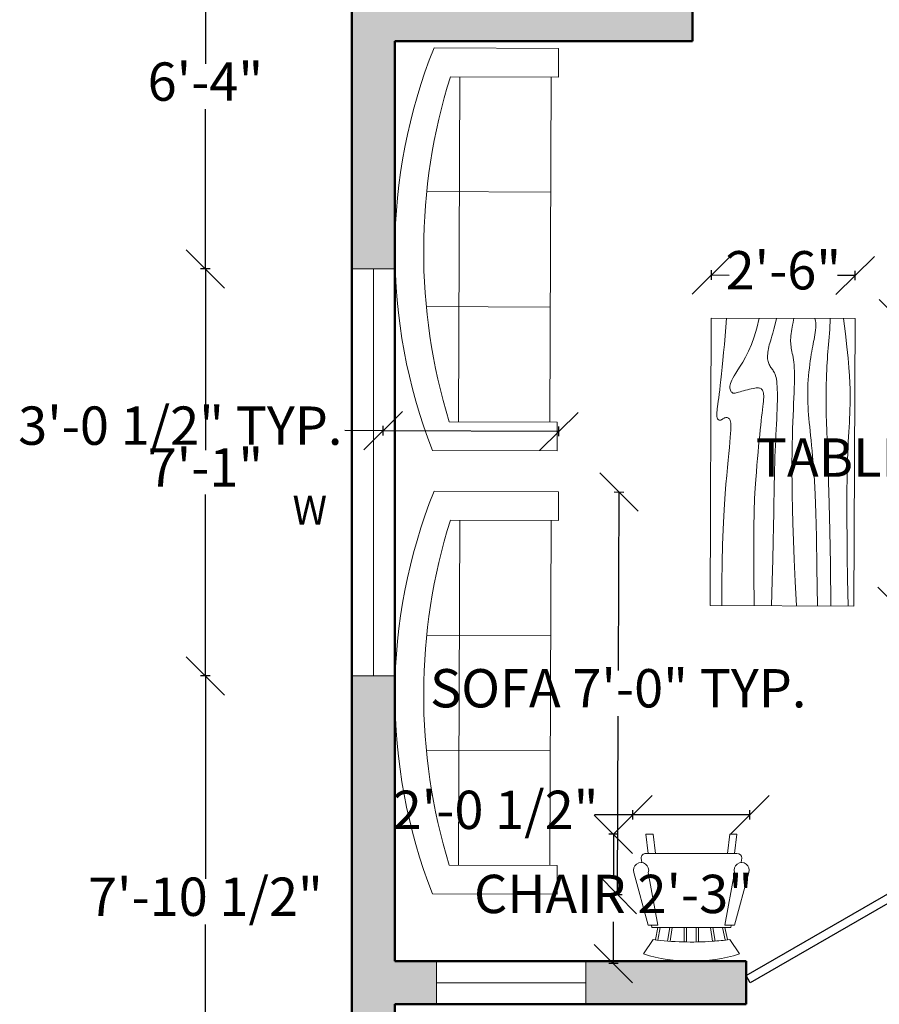
# Model space of a CAD drawing. Units: inches. Extents: x 3121 to 3511, y 1323 to 1998.
# Tile 7 of 10: x 3121 to 3300, y 1539 to 1744. Entities that reach past the tile are written whole.
import ezdxf

# ---------------------------------------------------------------- set-up
doc = ezdxf.new("R2010")
doc.units = ezdxf.units.IN
for name, color, linetype, lineweight in [('A-ANNO-DIMS', 2, 'Continuous', 18), ('A-ANNO-TEXT', 7, 'Continuous', 18), ('A-DOOR', 3, 'Continuous', 25), ('A-FURN', 8, 'Continuous', 18), ('A-GLAZ', 4, 'Continuous', 18), ('A-WALL', 7, 'Continuous', 50), ('A-WALL-PATT', 3, 'Continuous', 13)]:
    doc.layers.add(name, color=color, linetype=linetype, lineweight=lineweight)
doc.styles.get("Standard").update_dxf_attribs({"font": 'arial.ttf'})
doc.dimstyles.new('ISO-25', dxfattribs={"dimtxt": 8, "dimasz": 8, "dimexe": 1, "dimexo": 1, "dimtad": 0, "dimtih": 1, "dimtoh": 1, "dimlunit": 3, "dimtxsty": 'Standard', "dimblk": 'OBLIQUE', "dimcen": 2.5, "dimclrt": 1, "dimadec": 0, "dimazin": 0, "dimtfac": 1, "dimtmove": 0, "dimatfit": 3, "dimfxl": 1, "dimfxlon": 1, "dimarcsym": 0})

# ---------------------------------------------------------------- blocks, each defined once
blk = doc.blocks.new('Chair - Rocking')
for p, q in [((-8, -4.5), (-10, -1.5)), ((8, -4.5), (10, -1.5)), ((-1.5, -4.05012), (-1.5, -7)), ((-1, -7), (-1, -4.05012)), ((1, -7), (1, -4.04655)), ((1.5, -4.05012), (1.5, -7)), ((-7.5, -4.5), (-7, -7)), ((-6.5, -7), (-7.02225, -4.43)), ((-4.5, -7), (-4.96674, -4.19951)), ((-4, -7), (-4.40532, -4.16272)), ((4, -7), (4.40187, -4.18694)), ((4.5, -7), (4.96761, -4.19437)), ((6.5, -7), (7, -4.4057)), ((7.5, -4.5), (7, -7)), ((-9, -7.5), (-12, -18.49999)), ((-7, -7.5), (-9, -7.5)), ((-9, -18.49999), (-7, -7.5)), ((-8.23428, -6.99939), (-8.3093, -7.47958)), ((-8.23041, -7), (8.23915, -7)), ((7, -7.5), (9, -7.5)), ((9, -18.49999), (7, -7.5)), ((8.31071, -7.48854), (8.23449, -7.00073)), ((9, -7.5), (12, -18.49999)), ((-10.36644, -20.64523), (-10.5, -21.49999)), ((-9, -22.49999), (-9.5, -26.49999)), ((0, -22.49999), (-9.5, -22.49999)), ((-8, -26.49999), (-7.5, -22.49999)), ((0, -22.49999), (9.5, -22.49999)), ((8, -26.49999), (7.5, -22.49999)), ((9, -22.49999), (9.5, -26.49999)), ((10.5, -21.49999), (10.3575, -20.58798)), ((-9.5, -26.49999), (-8, -26.49999)), ((9.5, -26.49999), (8, -26.49999))]:
    blk.add_line(p, q)
for centre, radius, start, end in [((0, -34.08333), 34.08333, 72.93847, 107.0615), ((0, -68.25004), 64.25, 82.84733, 93.92211), ((0, -68.25004), 64.25, 93.92211, 97.15267), ((-10.5, -18.99999), 1.58114, 161.5651, 18.43495), ((10.5, -18.99999), 1.58114, 161.5651, 18.43495), ((-9.5, -21.49999), 1, 180, 270), ((9.5, -21.49999), 1, 270, 0)]:
    blk.add_arc(centre, radius, start, end)
blk = doc.blocks.new('Sofa - Roundback 7 ft.')
for p, q in [((-12.00002, -32.4421), (-12.00003, -6.5971)), ((11.99997, -32.4421), (11.99998, -6.5971)), ((-36.000027, -34), (-36.000027, -11.4696)), ((35.99998, -34), (35.99998, -11.4696)), ((-35.999844, -13.3819), (35.9998, -13.3819)), ((-36.000027, -32.4421), (35.99998, -32.4421))]:
    blk.add_line(p, q)
for points in [[(-36.000027, -34), (-42.000027, -34), (-42.000027, -8)], [(41.99998, -8), (41.99998, -34), (35.99998, -34)]]:
    blk.add_lwpolyline(points)
for centre, radius, start, end in [((0, -114.25), 114.25, 68.43141, 111.5686), ((-0.00001, -127.1968), 121.1968, 72.72033, 107.2797)]:
    blk.add_arc(centre, radius, start, end)
blk = doc.blocks.new('Table - Rectangular Woodgrain 60 x 30 in.')
for p, q in [((0, 0), (0, -30)), ((60, 0), (0, 0)), ((60, -30), (60, 0)), ((0, -30), (60, -30))]:
    blk.add_line(p, q)
for points in [[(0, -2.4), (4.8155, -2.418), (9.0302, -2.4688), (12.709, -2.5477), (15.9167, -2.65), (18.7181, -2.7711), (21.1781, -2.9063), (23.3616, -3.0508), (25.3333, -3.2), (27.1477, -3.3495), (28.8172, -3.4958), (30.3437, -3.636), (31.7291, -3.7667), (32.9756, -3.8849), (34.0849, -3.9875), (35.059, -4.0714), (35.9, -4.1334), (36.6114, -4.1711), (37.2041, -4.1854), (37.6906, -4.1779), (38.0833, -4.15), (38.3948, -4.1034), (38.6375, -4.0396), (38.8239, -3.9602), (38.9666, -3.8667), (39.0764, -3.7608), (39.1573, -3.6448), (39.2116, -3.521), (39.2416, -3.3917), (39.2498, -3.2593), (39.2385, -3.1261), (39.21, -2.9944), (39.1666, -2.8667), (39.111, -2.7447), (39.0468, -2.6281), (38.978, -2.5163), (38.9083, -2.4083), (38.8418, -2.3035), (38.7823, -2.201), (38.7337, -2.1001), (38.7, -2), (38.6844, -1.9003), (38.6875, -1.8021), (38.7094, -1.707), (38.75, -1.6167), (38.8094, -1.5326), (38.8875, -1.4563), (38.9844, -1.3893), (39.1, -1.3333), (39.2351, -1.2896), (39.3937, -1.2583), (39.5804, -1.2396), (39.8, -1.2333), (40.057, -1.2396), (40.3562, -1.2583), (40.7023, -1.2896), (41.1, -1.3333), (41.5547, -1.3895), (42.0755, -1.4573), (42.6721, -1.5361), (43.3542, -1.625), (44.1316, -1.7233), (45.014, -1.8302), (46.0114, -1.9449), (47.1333, -2.0667), (48.3862, -2.1947), (49.7625, -2.3281), (51.2513, -2.4663), (52.8416, -2.6083), (54.5226, -2.7535), (56.2833, -2.9011), (58.1127, -3.0501), (60, -3.2)], [(0, -9.2), (6.5759, -9.0858), (11.9385, -9.0365), (16.2527, -9.0418), (19.6833, -9.0917), (22.3952, -9.1759), (24.5531, -9.2844), (26.322, -9.4069), (27.8666, -9.5333), (29.3241, -9.6553), (30.7203, -9.7719), (32.0532, -9.8837), (33.3208, -9.9917), (34.5213, -10.0965), (35.6526, -10.199), (36.7128, -10.2999), (37.7, -10.4), (38.6129, -10.4996), (39.4531, -10.5969), (40.223, -10.6895), (40.925, -10.775), (41.5613, -10.8512), (42.1344, -10.9156), (42.6465, -10.966), (43.1, -11), (43.4976, -11.0158), (43.8437, -11.0136), (44.143, -10.9942), (44.4, -10.9583), (44.6195, -10.9069), (44.8062, -10.8406), (44.9648, -10.7603), (45.1, -10.6667), (45.2155, -10.5598), (45.3114, -10.4365), (45.3871, -10.2929), (45.4416, -10.125), (45.4743, -9.929), (45.4844, -9.7011), (45.4709, -9.4371), (45.4333, -9.1333), (45.3716, -8.7883), (45.2896, -8.4104), (45.1919, -8.0107), (45.0833, -7.6), (44.9685, -7.1893), (44.8521, -6.7896), (44.7388, -6.4117), (44.6333, -6.0667), (44.54, -5.7628), (44.4614, -5.4979), (44.4001, -5.2675), (44.3583, -5.0667), (44.3384, -4.8909), (44.3427, -4.7354), (44.3736, -4.5956), (44.4333, -4.4667), (44.5236, -4.3453), (44.6427, -4.2333), (44.7884, -4.1339), (44.9583, -4.05), (45.1501, -3.9849), (45.3614, -3.9417), (45.59, -3.9234), (45.8333, -3.9333), (46.0915, -3.9749), (46.3734, -4.0531), (46.6906, -4.1736), (47.0542, -4.3417), (47.4756, -4.5629), (47.9661, -4.8427), (48.5372, -5.1866), (49.2, -5.6), (49.9676, -6.0844), (50.8594, -6.625), (51.8965, -7.2031), (53.1, -7.8), (54.491, -8.3969), (56.0906, -8.975), (57.9199, -9.5156), (60, -10)], [(0, -12.8), (5.1847, -12.9322), (9.6213, -13.0323), (13.3963, -13.1059), (16.5958, -13.1583), (19.3063, -13.1952), (21.614, -13.2219), (23.6054, -13.2439), (25.3666, -13.2667), (26.9728, -13.2947), (28.4531, -13.3281), (29.8256, -13.3663), (31.1083, -13.4083), (32.3191, -13.4535), (33.476, -13.501), (34.597, -13.5501), (35.7, -13.6), (36.7984, -13.6497), (37.8875, -13.6979), (38.9578, -13.743), (40, -13.7833), (41.0047, -13.8174), (41.9625, -13.8438), (42.864, -13.8607), (43.7, -13.8667), (44.4631, -13.8604), (45.1552, -13.8417), (45.7801, -13.8104), (46.3416, -13.7667), (46.8439, -13.7104), (47.2906, -13.6417), (47.6858, -13.5604), (48.0333, -13.4667), (48.3375, -13.3608), (48.6042, -13.2448), (48.8396, -13.121), (49.05, -12.9917), (49.2417, -12.8593), (49.4208, -12.7261), (49.5937, -12.5944), (49.7667, -12.4667), (49.9452, -12.3451), (50.1323, -12.2313), (50.3303, -12.1268), (50.5416, -12.0333), (50.7686, -11.9524), (51.0135, -11.8854), (51.2788, -11.8341), (51.5666, -11.8), (51.8785, -11.7843), (52.2116, -11.7865), (52.562, -11.8059), (52.926, -11.8417), (53.2998, -11.8931), (53.6795, -11.9594), (54.0614, -12.0397), (54.4416, -12.1333), (54.8223, -12.2401), (55.2293, -12.3625), (55.6942, -12.5037), (56.2489, -12.6667), (56.9251, -12.8547), (57.7545, -13.0708), (58.7689, -13.3182), (60, -13.6)], [(0, -18), (5.124, -17.7273), (9.6609, -17.5057), (13.6705, -17.3303), (17.2125, -17.1958), (20.3467, -17.0973), (23.1328, -17.0297), (25.6307, -16.9878), (27.9, -16.9667), (29.9928, -16.9617), (31.9302, -16.9703), (33.7254, -16.9907), (35.3917, -17.0208), (36.9423, -17.0588), (38.3906, -17.1026), (39.7499, -17.1503), (41.0333, -17.2), (42.2519, -17.2496), (43.4073, -17.2969), (44.4986, -17.3395), (45.525, -17.375), (46.4858, -17.4012), (47.3802, -17.4156), (48.2074, -17.416), (48.9667, -17.4), (49.6583, -17.3662), (50.2872, -17.3167), (50.8595, -17.2547), (51.3812, -17.1833), (51.8584, -17.1057), (52.2971, -17.025), (52.7034, -16.9443), (53.0833, -16.8667), (53.443, -16.7951), (53.789, -16.7313), (54.128, -16.6768), (54.4666, -16.6334), (54.8115, -16.6024), (55.1693, -16.5854), (55.5465, -16.5841), (55.95, -16.6), (56.3828, -16.6337), (56.8346, -16.6823), (57.2915, -16.7418), (57.7396, -16.8084), (58.165, -16.878), (58.5539, -16.9469), (58.8924, -17.0111), (59.1666, -17.0667), (59.3679, -17.1107), (59.5078, -17.1438), (59.6032, -17.1675), (59.6708, -17.1833), (59.7275, -17.193), (59.7901, -17.1979), (59.8753, -17.1998), (60, -17.2)], [(0, -22.4), (8.0098, -22.2501), (14.4094, -22.1011), (19.4168, -21.9535), (23.25, -21.8083), (26.1269, -21.6663), (28.2656, -21.5281), (29.884, -21.3947), (31.2, -21.2667), (32.3967, -21.1448), (33.5172, -21.0292), (34.5697, -20.9198), (35.5625, -20.8167), (36.5037, -20.7198), (37.4015, -20.6292), (38.2642, -20.5448), (39.1, -20.4667), (39.9164, -20.3951), (40.7187, -20.3313), (41.5117, -20.2768), (42.3, -20.2333), (43.0883, -20.2024), (43.8812, -20.1854), (44.6836, -20.1841), (45.5, -20.2), (46.3328, -20.234), (47.1747, -20.2844), (48.0163, -20.3488), (48.8479, -20.425), (49.66, -20.5106), (50.4429, -20.6031), (51.1872, -20.7004), (51.8833, -20.8), (52.5246, -20.8999), (53.1166, -20.9995), (53.6681, -21.0983), (54.1875, -21.1958), (54.6834, -21.2919), (55.1646, -21.3859), (55.6394, -21.4777), (56.1167, -21.5667), (56.6028, -21.6515), (57.0961, -21.7266), (57.5929, -21.7852), (58.0896, -21.8208), (58.5823, -21.8268), (59.0674, -21.7964), (59.5412, -21.723), (60, -21.6)], [(0, -25.2), (8.6355, -25.0504), (15.7026, -24.9031), (21.4049, -24.7606), (25.9458, -24.625), (29.529, -24.4988), (32.3578, -24.3844), (34.6359, -24.284), (36.5667, -24.2), (38.3213, -24.1341), (39.9417, -24.0854), (41.437, -24.0523), (42.8167, -24.0333), (44.0901, -24.0268), (45.2667, -24.0313), (46.3557, -24.0451), (47.3667, -24.0667), (48.309, -24.0947), (49.1928, -24.1287), (50.0284, -24.168), (50.826, -24.2125), (51.5959, -24.2617), (52.3483, -24.3151), (53.0935, -24.3725), (53.8417, -24.4334), (54.6009, -24.497), (55.3699, -24.561), (56.1454, -24.6226), (56.9239, -24.6792), (57.7021, -24.7279), (58.4764, -24.7662), (59.2435, -24.7911), (60, -24.8)], [(0, -28.8), (5.6867, -28.6681), (10.45, -28.5698), (14.407, -28.5012), (17.675, -28.4584), (20.3711, -28.4374), (22.6125, -28.4344), (24.5164, -28.4455), (26.2, -28.4667), (27.762, -28.4947), (29.2276, -28.5281), (30.6033, -28.5663), (31.8958, -28.6084), (33.1118, -28.6535), (34.2578, -28.7011), (35.3405, -28.7501), (36.3666, -28.8), (37.3443, -28.8497), (38.288, -28.8974), (39.2137, -28.9412), (40.1375, -28.9792), (41.0753, -29.0093), (42.0432, -29.0297), (43.0572, -29.0384), (44.1333, -29.0333), (45.2936, -29.0114), (46.5843, -28.9641), (48.0579, -28.8816), (49.7666, -28.7542), (51.7629, -28.5721), (54.0989, -28.3255), (56.8272, -28.0048), (60, -27.6)]]:
    blk.add_lwpolyline(points)
blk = doc.blocks.new('*U11')
for p, q in [((0, 0), (0, -6)), ((40, 0), (40, -6))]:
    blk.add_line(p, q)
blk.add_lwpolyline([(0, 0), (34.64, 20), (35.52, 18.48), (0.87, -1.52)], close=True)
blk.add_arc((0, 0), 40, 0, 30)
blk = doc.blocks.new('_Oblique')
at = {"color": 0, "linetype": 'ByBlock', "lineweight": -2}
blk.add_line((-0.5, -0.5), (0.5, 0.5), dxfattribs=at)
blk = doc.blocks.new('*D21')
at = {"layer": 'A-ANNO-DIMS', "color": 0, "lineweight": -2, "transparency": 16777216}
for p, q in [((3244.67, 1645.71), (3246.67, 1645.7)), ((3245.67, 1645.71), (3245.54, 1608.47)), ((3245.36, 1561.71), (3245.5, 1598.94)), ((3244.36, 1561.71), (3246.36, 1561.7))]:
    blk.add_line(p, q, dxfattribs=at)
at = {"layer": 'Defpoints', "color": 0, "transparency": 16777216}
for p in [(3233.07, 1645.75), (3245.67, 1645.71), (3232.76, 1561.76)]:
    blk.add_point(p, dxfattribs=at)
at = {"layer": 'A-ANNO-DIMS', "color": 0, "lineweight": -2, "transparency": 16777216, "xscale": 8, "yscale": 8, "zscale": 8}
for p, rotation in [((3245.67, 1645.71), 89.78583340711933), ((3245.36, 1561.71), 269.7858334071193)]:
    blk.add_blockref('_Oblique', p, dxfattribs=dict(at, rotation=rotation))
at = {"layer": 'A-ANNO-DIMS', "color": 1, "transparency": 16777216, "insert": (3245.52, 1603.71), "char_height": 8, "attachment_point": 5}
blk.add_mtext('SOFA 7\'-0" TYP.', dxfattribs=at)
blk = doc.blocks.new('*D22')
at = {"layer": 'A-ANNO-DIMS', "color": 0, "lineweight": -2, "transparency": 16777216}
for p, q in [((3196.46, 1658.49), (3188.46, 1658.52)), ((3196.45, 1657.49), (3196.46, 1659.49)), ((3233.12, 1658.35), (3196.46, 1658.49)), ((3233.12, 1657.35), (3233.13, 1659.35))]:
    blk.add_line(p, q, dxfattribs=at)
at = {"layer": 'Defpoints', "color": 0, "transparency": 16777216}
for p in [(3196.46, 1658.49), (3196.41, 1645.89), (3233.07, 1645.75)]:
    blk.add_point(p, dxfattribs=at)
at = {"layer": 'A-ANNO-DIMS', "color": 0, "lineweight": -2, "transparency": 16777216, "xscale": 8, "yscale": 8, "zscale": 8}
for p, rotation in [((3196.46, 1658.49), 179.7858334071193), ((3233.12, 1658.35), 359.7858334071194)]:
    blk.add_blockref('_Oblique', p, dxfattribs=dict(at, rotation=rotation))
at = {"layer": 'A-ANNO-DIMS', "color": 1, "transparency": 16777216, "insert": (3154.13, 1658.52), "char_height": 8, "attachment_point": 5}
blk.add_mtext('3\'-0 1/2" TYP.', dxfattribs=at)
blk = doc.blocks.new('*D25')
at = {"layer": 'A-ANNO-DIMS', "color": 0, "lineweight": -2, "transparency": 16777216}
for p, q in [((3245.53, 1574.28), (3243.53, 1574.28)), ((3244.53, 1574.28), (3244.53, 1565.55)), ((3244.53, 1547.28), (3244.53, 1556.02)), ((3245.53, 1547.28), (3243.53, 1547.28))]:
    blk.add_line(p, q, dxfattribs=at)
at = {"layer": 'Defpoints', "color": 0, "transparency": 16777216}
for p in [(3248.58, 1574.28), (3244.53, 1547.28), (3248.58, 1547.28)]:
    blk.add_point(p, dxfattribs=at)
at = {"layer": 'A-ANNO-DIMS', "color": 0, "lineweight": -2, "transparency": 16777216, "xscale": 8, "yscale": 8, "zscale": 8}
for p, rotation in [((3244.53, 1574.28), 90), ((3244.53, 1547.28), 270)]:
    blk.add_blockref('_Oblique', p, dxfattribs=dict(at, rotation=rotation))
at = {"layer": 'A-ANNO-DIMS', "color": 1, "transparency": 16777216, "insert": (3244.53, 1560.78), "char_height": 8, "attachment_point": 5}
blk.add_mtext('CHAIR 2\'-3"', dxfattribs=at)
blk = doc.blocks.new('*D26')
at = {"layer": 'A-ANNO-DIMS', "color": 0, "lineweight": -2, "transparency": 16777216}
for p, q in [((3248.58, 1578.33), (3240.58, 1578.33)), ((3248.58, 1577.33), (3248.58, 1579.33)), ((3273.01, 1578.33), (3248.58, 1578.33)), ((3273.01, 1577.33), (3273.01, 1579.33))]:
    blk.add_line(p, q, dxfattribs=at)
at = {"layer": 'Defpoints', "color": 0, "transparency": 16777216}
for p in [(3248.58, 1578.33), (3248.58, 1574.28), (3273.01, 1574.28)]:
    blk.add_point(p, dxfattribs=at)
at = {"layer": 'A-ANNO-DIMS', "color": 0, "lineweight": -2, "transparency": 16777216, "xscale": 8, "yscale": 8, "zscale": 8, "rotation": 180}
blk.add_blockref('_Oblique', (3248.58, 1578.33), dxfattribs=at)
at = {"layer": 'A-ANNO-DIMS', "color": 0, "lineweight": -2, "transparency": 16777216, "xscale": 8, "yscale": 8, "zscale": 8}
blk.add_blockref('_Oblique', (3273.01, 1578.33), dxfattribs=at)
at = {"layer": 'A-ANNO-DIMS', "color": 1, "transparency": 16777216, "insert": (3219.93, 1578.33), "char_height": 8, "attachment_point": 5}
blk.add_mtext('2\'-0 1/2"', dxfattribs=at)
blk = doc.blocks.new('*D29')
at = {"layer": 'A-ANNO-DIMS', "color": 0, "lineweight": -2, "transparency": 16777216}
for p, q in [((3302.93, 1681.86), (3304.93, 1681.86)), ((3303.93, 1681.86), (3303.84, 1656.57)), ((3303.71, 1621.86), (3303.8, 1647.15)), ((3302.71, 1621.86), (3304.71, 1621.86))]:
    blk.add_line(p, q, dxfattribs=at)
at = {"layer": 'Defpoints', "color": 0, "transparency": 16777216}
for p in [(3294.93, 1681.89), (3303.93, 1681.86), (3294.71, 1621.89)]:
    blk.add_point(p, dxfattribs=at)
at = {"layer": 'A-ANNO-DIMS', "color": 0, "lineweight": -2, "transparency": 16777216, "xscale": 8, "yscale": 8, "zscale": 8}
for p, rotation in [((3303.93, 1681.86), 89.78583340711918), ((3303.71, 1621.86), 269.7858334071192)]:
    blk.add_blockref('_Oblique', p, dxfattribs=dict(at, rotation=rotation))
at = {"layer": 'A-ANNO-DIMS', "color": 1, "transparency": 16777216, "insert": (3303.82, 1651.86), "char_height": 8, "attachment_point": 5}
blk.add_mtext('TABLE 5\'-0"', dxfattribs=at)
blk = doc.blocks.new('*D30')
at = {"layer": 'A-ANNO-DIMS', "color": 0, "lineweight": -2, "transparency": 16777216}
for p, q in [((3264.96, 1690), (3264.97, 1692)), ((3294.96, 1689.89), (3294.97, 1691.89)), ((3264.97, 1691), (3268.64, 1690.99)), ((3294.97, 1690.89), (3291.29, 1690.91))]:
    blk.add_line(p, q, dxfattribs=at)
at = {"layer": 'Defpoints', "color": 0, "transparency": 16777216}
for p in [(3264.97, 1691), (3264.93, 1682), (3294.93, 1681.89)]:
    blk.add_point(p, dxfattribs=at)
at = {"layer": 'A-ANNO-DIMS', "color": 0, "lineweight": -2, "transparency": 16777216, "xscale": 8, "yscale": 8, "zscale": 8}
for p, rotation in [((3264.97, 1691), 179.7858334071191), ((3294.97, 1690.89), 359.7858334071192)]:
    blk.add_blockref('_Oblique', p, dxfattribs=dict(at, rotation=rotation))
at = {"layer": 'A-ANNO-DIMS', "color": 1, "transparency": 16777216, "insert": (3279.97, 1690.95), "char_height": 8, "attachment_point": 5}
blk.add_mtext('2\'-6"', dxfattribs=at)
blk = doc.blocks.new('*D37')
at = {"layer": 'A-ANNO-DIMS', "color": 0, "lineweight": -2, "transparency": 16777216}
for p, q in [((3160.37, 1607.33), (3158.37, 1607.33)), ((3159.37, 1607.33), (3159.37, 1564.96)), ((3159.37, 1513.07), (3159.37, 1555.44)), ((3160.37, 1513.07), (3158.37, 1513.07))]:
    blk.add_line(p, q, dxfattribs=at)
at = {"layer": 'Defpoints', "color": 0, "transparency": 16777216}
for p in [(3159.37, 1607.33), (3189.92, 1607.33), (3189.92, 1513.07)]:
    blk.add_point(p, dxfattribs=at)
at = {"layer": 'A-ANNO-DIMS', "color": 0, "lineweight": -2, "transparency": 16777216, "xscale": 8, "yscale": 8, "zscale": 8}
for p, rotation in [((3159.37, 1607.33), 90), ((3159.37, 1513.07), 270)]:
    blk.add_blockref('_Oblique', p, dxfattribs=dict(at, rotation=rotation))
at = {"layer": 'A-ANNO-DIMS', "color": 1, "transparency": 16777216, "insert": (3159.37, 1560.2), "char_height": 8, "attachment_point": 5}
blk.add_mtext('7\'-10 1/2"', dxfattribs=at)
blk = doc.blocks.new('*D38')
at = {"layer": 'A-ANNO-DIMS', "color": 0, "lineweight": -2, "transparency": 16777216}
for p, q in [((3160.37, 1692.28), (3158.37, 1692.28)), ((3159.37, 1692.28), (3159.37, 1654.44)), ((3159.37, 1607.33), (3159.37, 1645.16)), ((3160.37, 1607.33), (3158.37, 1607.33))]:
    blk.add_line(p, q, dxfattribs=at)
at = {"layer": 'Defpoints', "color": 0, "transparency": 16777216}
for p in [(3159.37, 1692.28), (3189.92, 1692.28), (3189.92, 1607.33)]:
    blk.add_point(p, dxfattribs=at)
at = {"layer": 'A-ANNO-DIMS', "color": 0, "lineweight": -2, "transparency": 16777216, "xscale": 8, "yscale": 8, "zscale": 8}
for p, rotation in [((3159.37, 1692.28), 90), ((3159.37, 1607.33), 270)]:
    blk.add_blockref('_Oblique', p, dxfattribs=dict(at, rotation=rotation))
at = {"layer": 'A-ANNO-DIMS', "color": 1, "transparency": 16777216, "insert": (3159.37, 1649.8), "char_height": 8, "attachment_point": 5}
blk.add_mtext('7\'-1"', dxfattribs=at)
blk = doc.blocks.new('*D39')
at = {"layer": 'A-ANNO-DIMS', "color": 0, "lineweight": -2, "transparency": 16777216}
for p, q in [((3160.37, 1768.39), (3158.37, 1768.39)), ((3159.37, 1768.39), (3159.37, 1735.04)), ((3159.37, 1692.28), (3159.37, 1725.62)), ((3160.37, 1692.28), (3158.37, 1692.28))]:
    blk.add_line(p, q, dxfattribs=at)
at = {"layer": 'Defpoints', "color": 0, "transparency": 16777216}
for p in [(3159.37, 1768.39), (3189.92, 1768.39), (3189.92, 1692.28)]:
    blk.add_point(p, dxfattribs=at)
at = {"layer": 'A-ANNO-DIMS', "color": 0, "lineweight": -2, "transparency": 16777216, "xscale": 8, "yscale": 8, "zscale": 8}
for p, rotation in [((3159.37, 1768.39), 90), ((3159.37, 1692.28), 270)]:
    blk.add_blockref('_Oblique', p, dxfattribs=dict(at, rotation=rotation))
at = {"layer": 'A-ANNO-DIMS', "color": 1, "transparency": 16777216, "insert": (3159.37, 1730.33), "char_height": 8, "attachment_point": 5}
blk.add_mtext('6\'-4"', dxfattribs=at)
blk = doc.blocks.new('*D53')
at = {"layer": 'A-ANNO-DIMS', "color": 0, "lineweight": -2, "transparency": 16777216}
for p, q in [((3274.02, 1336.37), (3274.02, 1334.37)), ((3310.02, 1336.37), (3310.02, 1334.37)), ((3274.02, 1335.37), (3280.77, 1335.37)), ((3310.02, 1335.37), (3303.28, 1335.37))]:
    blk.add_line(p, q, dxfattribs=at)
at = {"layer": 'Defpoints', "color": 0, "transparency": 16777216}
for p in [(3274.02, 1946.78), (3310.02, 1946.78), (3310.02, 1335.37)]:
    blk.add_point(p, dxfattribs=at)
at = {"layer": 'A-ANNO-DIMS', "color": 0, "lineweight": -2, "transparency": 16777216, "xscale": 8, "yscale": 8, "zscale": 8, "rotation": 180}
blk.add_blockref('_Oblique', (3274.02, 1335.37), dxfattribs=at)
at = {"layer": 'A-ANNO-DIMS', "color": 0, "lineweight": -2, "transparency": 16777216, "xscale": 8, "yscale": 8, "zscale": 8}
blk.add_blockref('_Oblique', (3310.02, 1335.37), dxfattribs=at)
at = {"layer": 'A-ANNO-DIMS', "color": 1, "transparency": 16777216, "insert": (3292.02, 1335.37), "char_height": 8, "attachment_point": 5}
blk.add_mtext('3\'-0"', dxfattribs=at)
blk = doc.blocks.new('*D58')
at = {"layer": 'A-ANNO-DIMS', "color": 0, "lineweight": -2, "transparency": 16777216}
for p, q in [((3209.89, 1985.33), (3209.89, 1987.33)), ((3311.33, 1985.33), (3311.33, 1987.33)), ((3209.89, 1986.33), (3240.03, 1986.33)), ((3311.33, 1986.33), (3281.19, 1986.33))]:
    blk.add_line(p, q, dxfattribs=at)
at = {"layer": 'Defpoints', "color": 0, "transparency": 16777216}
for p in [(3311.33, 1986.33), (3209.89, 1424.78), (3311.33, 1424.78)]:
    blk.add_point(p, dxfattribs=at)
at = {"layer": 'A-ANNO-DIMS', "color": 0, "lineweight": -2, "transparency": 16777216, "xscale": 8, "yscale": 8, "zscale": 8, "rotation": 180}
blk.add_blockref('_Oblique', (3209.89, 1986.33), dxfattribs=at)
at = {"layer": 'A-ANNO-DIMS', "color": 0, "lineweight": -2, "transparency": 16777216, "xscale": 8, "yscale": 8, "zscale": 8}
blk.add_blockref('_Oblique', (3311.33, 1986.33), dxfattribs=at)
at = {"layer": 'A-ANNO-DIMS', "color": 1, "transparency": 16777216, "insert": (3260.61, 1986.33), "char_height": 8, "attachment_point": 5}
blk.add_mtext('8\'-5 1/2"', dxfattribs=at)
blk = doc.blocks.new('*D73')
at = {"layer": 'A-ANNO-DIMS', "color": 0, "lineweight": -2, "transparency": 16777216}
for p, q in [((3261.02, 1336.37), (3261.02, 1334.37)), ((3301.03, 1336.37), (3301.03, 1334.37)), ((3261.02, 1335.37), (3269.77, 1335.37)), ((3301.03, 1335.37), (3292.28, 1335.37))]:
    blk.add_line(p, q, dxfattribs=at)
at = {"layer": 'Defpoints', "color": 0, "transparency": 16777216}
for p in [(3261.02, 1739.78), (3301.03, 1739.78), (3301.03, 1335.37)]:
    blk.add_point(p, dxfattribs=at)
at = {"layer": 'A-ANNO-DIMS', "color": 0, "lineweight": -2, "transparency": 16777216, "xscale": 8, "yscale": 8, "zscale": 8, "rotation": 180}
blk.add_blockref('_Oblique', (3261.02, 1335.37), dxfattribs=at)
at = {"layer": 'A-ANNO-DIMS', "color": 0, "lineweight": -2, "transparency": 16777216, "xscale": 8, "yscale": 8, "zscale": 8}
blk.add_blockref('_Oblique', (3301.03, 1335.37), dxfattribs=at)
at = {"layer": 'A-ANNO-DIMS', "color": 1, "transparency": 16777216, "insert": (3281.02, 1335.37), "char_height": 8, "attachment_point": 5}
blk.add_mtext('3\'-4"', dxfattribs=at)

msp = doc.modelspace()

# ---------------------------------------------------------------- hatches: boundary and pattern name
at = {"layer": 'A-WALL-PATT'}
h = msp.add_hatch(color=256, dxfattribs=at)
h.dxf.hatch_style = 1
h.paths.add_polyline_path([(3274.023, 1955.784), (3189.918, 1955.784), (3189.918, 1910.219), (3198.918, 1910.219), (3198.918, 1946.784), (3259.023, 1946.784), (3259.023, 1921.61), (3261.023, 1921.61), (3261.023, 1946.784), (3274.023, 1946.784)])
h.paths.add_polyline_path([(3327.918, 1946.784), (3334.156, 1946.784), (3334.156, 1955.784), (3310.023, 1955.784), (3310.023, 1946.784), (3318.918, 1946.784), (3318.918, 1929.796), (3311.644, 1929.796), (3311.644, 1927.007), (3324.033, 1927.007), (3324.033, 1871.381), (3311.644, 1871.381), (3311.644, 1868.381), (3318.918, 1868.381), (3318.918, 1853.784), (3327.918, 1853.784)])
h.paths.add_polyline_path([(3456.918, 1955.784), (3384.562, 1955.784), (3384.562, 1946.784), (3447.918, 1946.784), (3447.918, 1877.779), (3456.918, 1877.779)])
h.paths.add_polyline_path([(3456.918, 1835.782), (3447.918, 1835.782), (3447.918, 1814.784), (3414.918, 1814.784), (3414.918, 1803.784), (3447.918, 1803.784), (3447.918, 1793.443), (3456.918, 1793.443)])
h.paths.add_polyline_path([(3456.918, 1558.434), (3447.918, 1558.434), (3447.918, 1547.784), (3375.918, 1547.784), (3375.918, 1598.784), (3378.918, 1598.784), (3378.918, 1602.284), (3375.918, 1602.284), (3375.918, 1674.284), (3369.918, 1674.284), (3369.918, 1547.784), (3364.418, 1547.784), (3364.418, 1538.784), (3447.918, 1538.784), (3447.918, 1512.628), (3456.918, 1512.628)])
h.paths.add_polyline_path([(3456.918, 1460.558), (3447.918, 1460.558), (3447.918, 1424.784), (3412.543, 1424.784), (3412.543, 1415.784), (3456.918, 1415.784)])
h.paths.add_polyline_path([(3358.149, 1424.784), (3322.918, 1424.784), (3322.918, 1538.784), (3328.418, 1538.784), (3328.418, 1547.784), (3308.208, 1547.784), (3308.208, 1538.784), (3318.918, 1538.784), (3318.918, 1424.784), (3311.328, 1424.784), (3311.328, 1415.784), (3358.149, 1415.784)])
h.paths.add_polyline_path([(3207.562, 1547.784), (3198.918, 1547.784), (3198.918, 1607.327), (3189.918, 1607.327), (3189.918, 1513.073), (3198.918, 1513.073), (3198.918, 1538.784), (3207.562, 1538.784)])
h.paths.add_polyline_path([(3198.918, 1461.548), (3189.918, 1461.548), (3189.918, 1415.784), (3209.892, 1415.784), (3209.892, 1424.784), (3198.918, 1424.784)])
h.paths.add_polyline_path([(3272.208, 1547.784), (3238.766, 1547.784), (3238.766, 1538.784), (3272.208, 1538.784)])
h.paths.add_polyline_path([(3261.023, 1748.784), (3198.918, 1748.784), (3198.918, 1768.387), (3189.918, 1768.387), (3189.918, 1692.279), (3198.918, 1692.279), (3198.918, 1739.784), (3261.023, 1739.784)])
h.paths.add_polyline_path([(3198.918, 1856.171), (3189.918, 1856.171), (3189.918, 1808.331), (3198.918, 1808.331), (3198.918, 1821.074), (3261.023, 1821.074), (3261.023, 1862.309), (3259.023, 1862.309), (3259.023, 1825.074), (3198.918, 1825.074)])

# ---------------------------------------------------------------- linework, layer by layer
at = {"layer": 'A-GLAZ'}
for p, q in [((3198.918, 1692.279), (3189.918, 1692.279)), ((3194.418, 1692.279), (3194.418, 1607.327)), ((3189.918, 1607.327), (3198.918, 1607.327)), ((3207.562, 1547.784), (3207.562, 1538.784)), ((3238.766, 1547.784), (3238.766, 1538.784)), ((3207.562, 1543.284), (3238.766, 1543.284))]:
    msp.add_line(p, q, dxfattribs=at)
at = {"layer": 'A-WALL'}
for p, q in [((3189.918, 1955.784), (3189.918, 1415.784)), ((3261.023, 1748.784), (3261.023, 1739.784)), ((3198.918, 1739.784), (3198.918, 1547.784)), ((3261.023, 1739.784), (3198.918, 1739.784)), ((3272.208, 1547.784), (3198.918, 1547.784)), ((3272.208, 1547.784), (3272.208, 1538.784)), ((3198.918, 1538.784), (3198.918, 1424.784)), ((3272.208, 1538.784), (3198.918, 1538.784))]:
    msp.add_line(p, q, dxfattribs=at)

# ---------------------------------------------------------------- block references
at = {"layer": 'A-DOOR'}
msp.add_blockref('*U11', (3272.208, 1544.784), dxfattribs=at)
at = {"layer": 'A-FURN'}
for name, p, rotation in [('Sofa - Roundback 7 ft.', (3198.918, 1696.419), 89.78583340711928), ('Table - Rectangular Woodgrain 60 x 30 in.', (3264.709, 1622.005), 89.78583340711928), ('Sofa - Roundback 7 ft.', (3198.918, 1603.882), 89.78583340711928), ('Chair - Rocking', (3260.795, 1547.784), 180)]:
    msp.add_blockref(name, p, dxfattribs=dict(at, rotation=rotation))

# ---------------------------------------------------------------- texts
at = {"layer": 'A-ANNO-TEXT', "insert": (3174.942, 1644.909), "char_height": 6, "attachment_point": 1}
msp.add_mtext_dynamic_manual_height_columns('\\pxqc;W', width=12.42925, gutter_width=12.5, heights=[0], dxfattribs=at)

# ---------------------------------------------------------------- dimensions: what is measured, and where the dimension line sits
at = {"layer": 'A-ANNO-DIMS'}
for base, p1, p2, picture, middle in [((3311.328, 1986.334), (3209.892, 1424.784), (3311.328, 1424.784), '*D58', (3260.61, 1986.334)), ((3310.023, 1335.367), (3274.023, 1946.784), (3310.023, 1946.784), '*D53', (3292.023, 1335.367)), ((3301.026, 1335.367), (3261.023, 1739.784), (3301.026, 1739.784), '*D73', (3281.024, 1335.367))]:
    dim = msp.add_linear_dim(base=base, p1=p1, p2=p2, dimstyle='ISO-25', override={"dimdec": 1, "dimlfac": 1, "dimrnd": 0, "dimzin": 1, "dimdsep": 46, "dimlunit": 4, "dimfrac": 2}, dxfattribs=at)
    dim.commit()
    dim.dimension.update_dxf_attribs({"geometry": picture, "text_midpoint": middle})
for base, p1, p2, angle, picture, middle in [((3159.368, 1768.387), (3189.918, 1692.279), (3189.918, 1768.387), 90, '*D39', (3159.368, 1730.333)), ((3159.368, 1692.279), (3189.918, 1607.327), (3189.918, 1692.279), 90, '*D38', (3159.368, 1649.803)), ((3264.967, 1691.005), (3294.933, 1681.893), (3264.933, 1682.005), 179.78583, '*D30', (3279.967, 1690.949)), ((3159.368, 1607.327), (3189.918, 1513.073), (3189.918, 1607.327), 90, '*D37', (3159.368, 1560.2)), ((3248.578, 1578.334), (3273.013, 1574.284), (3248.578, 1574.284), 180, '*D26', (3219.931, 1578.334))]:
    dim = msp.add_linear_dim(base=base, p1=p1, p2=p2, angle=angle, dimstyle='ISO-25', override={"dimdec": 1, "dimlfac": 1, "dimrnd": 0, "dimzin": 1, "dimdsep": 46, "dimlunit": 4, "dimfrac": 2}, dxfattribs=at)
    dim.commit()
    dim.dimension.update_dxf_attribs({"geometry": picture, "text_midpoint": middle})
for base, p1, p2, angle, text, picture, middle in [((3303.933, 1681.859), (3294.709, 1621.893), (3294.933, 1681.893), 89.78583, 'TABLE <>', '*D29', (3303.821, 1651.859)), ((3196.455, 1658.492), (3233.075, 1645.755), (3196.408, 1645.892), 179.78583, '<> TYP.', '*D22', (3154.131, 1658.522)), ((3245.675, 1645.708), (3232.761, 1561.755), (3233.075, 1645.755), 89.78583, 'SOFA <> TYP.', '*D21', (3245.518, 1603.708)), ((3244.528, 1547.284), (3248.578, 1574.284), (3248.578, 1547.284), 270, 'CHAIR <>', '*D25', (3244.528, 1560.784))]:
    dim = msp.add_linear_dim(base=base, p1=p1, p2=p2, angle=angle, text=text, dimstyle='ISO-25', override={"dimdec": 1, "dimlfac": 1, "dimrnd": 0, "dimzin": 1, "dimdsep": 46, "dimlunit": 4, "dimfrac": 2}, dxfattribs=at)
    dim.commit()
    dim.dimension.update_dxf_attribs({"geometry": picture, "text_midpoint": middle})

doc.saveas('drawing.dxf')
